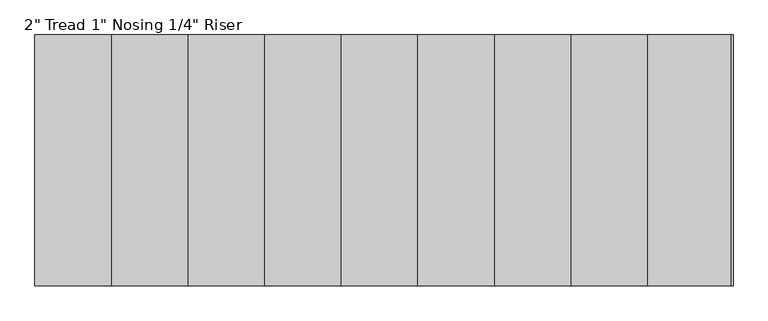
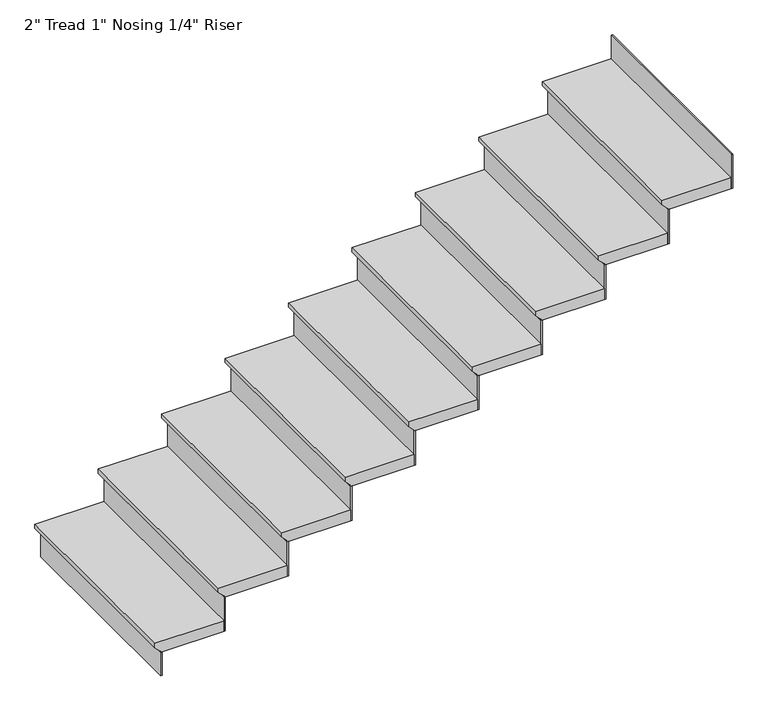
"""IFC4 building model written with IfcOpenShell, lengths in millimetres: stair flight geometry."""

from ifc_helpers import new_model, si_unit, origin, place, context, project, spatial, faceted_brep, source, transform, mapped, element, save


def stair_flight_ff2ce9cd(model_context):
    return source(origin(), model_context, "Body", "Brep", [
        faceted_brep([(-1591.1154463, -4737.3544725, 25744.17), (-1591.1154463, -4737.3544725, 25763.22), (-1591.1154463, -3822.9544725, 25763.22), (-1591.1154463, -3822.9544725, 25744.17), (-1565.7154463, -4737.3544725, 25718.77), (-1565.7154463, -3822.9544725, 25718.77), (-1286.3154463, -4737.3544725, 25763.22), (-1286.3154463, -3822.9544725, 25763.22), (-1565.7154463, -3822.9544725, 25712.42), (-1286.3154463, -3822.9544725, 25712.42), (-1286.3154463, -4737.3544725, 25712.42), (-1565.7154463, -4737.3544725, 25712.42)], [[[0, 1, 2, 3]], [[4, 0, 3, 5]], [[2, 1, 6, 7]], [[8, 9, 10, 11]], [[2, 7, 9, 8, 5, 3]], [[8, 11, 4, 5]], [[6, 1, 0, 4, 11, 10]], [[7, 6, 10, 9]]]),
        faceted_brep([(-1565.7154463, -4737.3544725, 25712.42), (-1565.7154463, -4737.3544725, 25603.2), (-1559.3654463, -4737.3544725, 25603.2), (-1559.3654463, -4737.3544725, 25712.42), (-1565.7154463, -3822.9544725, 25712.42), (-1559.3654463, -3822.9544725, 25712.42), (-1559.3654463, -3822.9544725, 25603.2), (-1565.7154463, -3822.9544725, 25603.2)], [[[0, 1, 2, 3]], [[4, 5, 6, 7]], [[1, 0, 4, 7]], [[2, 1, 7, 6]], [[3, 2, 6, 5]], [[0, 3, 5, 4]]]),
        faceted_brep([(-1286.3154463, -4737.3544725, 25872.44), (-1286.3154463, -4737.3544725, 25712.42), (-1279.9654463, -4737.3544725, 25712.42), (-1279.9654463, -4737.3544725, 25872.44), (-1286.3154463, -3822.9544725, 25872.44), (-1279.9654463, -3822.9544725, 25872.44), (-1279.9654463, -3822.9544725, 25712.42), (-1286.3154463, -3822.9544725, 25712.42)], [[[0, 1, 2, 3]], [[4, 5, 6, 7]], [[1, 0, 4, 7]], [[2, 1, 7, 6]], [[3, 2, 6, 5]], [[0, 3, 5, 4]]]),
        faceted_brep([(-1311.7154463, -3822.9544725, 25923.24), (-1311.7154463, -4737.3544725, 25923.24), (-1006.9154463, -4737.3544725, 25923.24), (-1006.9154463, -3822.9544725, 25923.24), (-1286.3154463, -3822.9544725, 25872.44), (-1006.9154463, -3822.9544725, 25872.44), (-1006.9154463, -4737.3544725, 25872.44), (-1286.3154463, -4737.3544725, 25872.44), (-1286.3154463, -3822.9544725, 25878.79), (-1311.7154463, -3822.9544725, 25904.19), (-1286.3154463, -4737.3544725, 25878.79), (-1311.7154463, -4737.3544725, 25904.19)], [[[0, 1, 2, 3]], [[4, 5, 6, 7]], [[0, 3, 5, 4, 8, 9]], [[4, 7, 10, 8]], [[2, 1, 11, 10, 7, 6]], [[3, 2, 6, 5]], [[11, 1, 0, 9]], [[10, 11, 9, 8]]]),
        faceted_brep([(-1006.9154463, -4737.3544725, 26032.46), (-1006.9154463, -4737.3544725, 25872.44), (-1000.5654463, -4737.3544725, 25872.44), (-1000.5654463, -4737.3544725, 26032.46), (-1006.9154463, -3822.9544725, 26032.46), (-1000.5654463, -3822.9544725, 26032.46), (-1000.5654463, -3822.9544725, 25872.44), (-1006.9154463, -3822.9544725, 25872.44)], [[[0, 1, 2, 3]], [[4, 5, 6, 7]], [[1, 0, 4, 7]], [[2, 1, 7, 6]], [[3, 2, 6, 5]], [[0, 3, 5, 4]]]),
        faceted_brep([(-1032.3154463, -3822.9544725, 26083.26), (-1032.3154463, -4737.3544725, 26083.26), (-727.5154463, -4737.3544725, 26083.26), (-727.5154463, -3822.9544725, 26083.26), (-1006.9154463, -3822.9544725, 26032.46), (-727.5154463, -3822.9544725, 26032.46), (-727.5154463, -4737.3544725, 26032.46), (-1006.9154463, -4737.3544725, 26032.46), (-1006.9154463, -3822.9544725, 26038.81), (-1032.3154463, -3822.9544725, 26064.21), (-1006.9154463, -4737.3544725, 26038.81), (-1032.3154463, -4737.3544725, 26064.21)], [[[0, 1, 2, 3]], [[4, 5, 6, 7]], [[0, 3, 5, 4, 8, 9]], [[4, 7, 10, 8]], [[2, 1, 11, 10, 7, 6]], [[3, 2, 6, 5]], [[11, 1, 0, 9]], [[10, 11, 9, 8]]]),
        faceted_brep([(-727.5154463, -4737.3544725, 26192.48), (-727.5154463, -4737.3544725, 26032.46), (-721.1654463, -4737.3544725, 26032.46), (-721.1654463, -4737.3544725, 26192.48), (-727.5154463, -3822.9544725, 26192.48), (-721.1654463, -3822.9544725, 26192.48), (-721.1654463, -3822.9544725, 26032.46), (-727.5154463, -3822.9544725, 26032.46)], [[[0, 1, 2, 3]], [[4, 5, 6, 7]], [[1, 0, 4, 7]], [[2, 1, 7, 6]], [[3, 2, 6, 5]], [[0, 3, 5, 4]]]),
        faceted_brep([(-752.9154463, -3822.9544725, 26243.28), (-752.9154463, -4737.3544725, 26243.28), (-448.1154463, -4737.3544725, 26243.28), (-448.1154463, -3822.9544725, 26243.28), (-727.5154463, -3822.9544725, 26192.48), (-448.1154463, -3822.9544725, 26192.48), (-448.1154463, -4737.3544725, 26192.48), (-727.5154463, -4737.3544725, 26192.48), (-727.5154463, -3822.9544725, 26198.83), (-752.9154463, -3822.9544725, 26224.23), (-727.5154463, -4737.3544725, 26198.83), (-752.9154463, -4737.3544725, 26224.23)], [[[0, 1, 2, 3]], [[4, 5, 6, 7]], [[0, 3, 5, 4, 8, 9]], [[4, 7, 10, 8]], [[2, 1, 11, 10, 7, 6]], [[3, 2, 6, 5]], [[11, 1, 0, 9]], [[10, 11, 9, 8]]]),
        faceted_brep([(-448.1154463, -4737.3544725, 26352.5), (-448.1154463, -4737.3544725, 26192.48), (-441.7654463, -4737.3544725, 26192.48), (-441.7654463, -4737.3544725, 26352.5), (-448.1154463, -3822.9544725, 26352.5), (-441.7654463, -3822.9544725, 26352.5), (-441.7654463, -3822.9544725, 26192.48), (-448.1154463, -3822.9544725, 26192.48)], [[[0, 1, 2, 3]], [[4, 5, 6, 7]], [[1, 0, 4, 7]], [[2, 1, 7, 6]], [[3, 2, 6, 5]], [[0, 3, 5, 4]]]),
        faceted_brep([(-473.5154463, -3822.9544725, 26403.3), (-473.5154463, -4737.3544725, 26403.3), (-168.7154463, -4737.3544725, 26403.3), (-168.7154463, -3822.9544725, 26403.3), (-448.1154463, -3822.9544725, 26352.5), (-168.7154463, -3822.9544725, 26352.5), (-168.7154463, -4737.3544725, 26352.5), (-448.1154463, -4737.3544725, 26352.5), (-448.1154463, -3822.9544725, 26358.85), (-473.5154463, -3822.9544725, 26384.25), (-448.1154463, -4737.3544725, 26358.85), (-473.5154463, -4737.3544725, 26384.25)], [[[0, 1, 2, 3]], [[4, 5, 6, 7]], [[0, 3, 5, 4, 8, 9]], [[4, 7, 10, 8]], [[2, 1, 11, 10, 7, 6]], [[3, 2, 6, 5]], [[11, 1, 0, 9]], [[10, 11, 9, 8]]]),
        faceted_brep([(-168.7154463, -4737.3544725, 26512.52), (-168.7154463, -4737.3544725, 26352.5), (-162.3654463, -4737.3544725, 26352.5), (-162.3654463, -4737.3544725, 26512.52), (-168.7154463, -3822.9544725, 26512.52), (-162.3654463, -3822.9544725, 26512.52), (-162.3654463, -3822.9544725, 26352.5), (-168.7154463, -3822.9544725, 26352.5)], [[[0, 1, 2, 3]], [[4, 5, 6, 7]], [[1, 0, 4, 7]], [[2, 1, 7, 6]], [[3, 2, 6, 5]], [[0, 3, 5, 4]]]),
        faceted_brep([(-194.1154463, -3822.9544725, 26563.32), (-194.1154463, -4737.3544725, 26563.32), (110.6845537, -4737.3544725, 26563.32), (110.6845537, -3822.9544725, 26563.32), (-168.7154463, -3822.9544725, 26512.52), (110.6845537, -3822.9544725, 26512.52), (110.6845537, -4737.3544725, 26512.52), (-168.7154463, -4737.3544725, 26512.52), (-168.7154463, -3822.9544725, 26518.87), (-194.1154463, -3822.9544725, 26544.27), (-168.7154463, -4737.3544725, 26518.87), (-194.1154463, -4737.3544725, 26544.27)], [[[0, 1, 2, 3]], [[4, 5, 6, 7]], [[0, 3, 5, 4, 8, 9]], [[4, 7, 10, 8]], [[2, 1, 11, 10, 7, 6]], [[3, 2, 6, 5]], [[11, 1, 0, 9]], [[10, 11, 9, 8]]]),
        faceted_brep([(110.6845537, -4737.3544725, 26672.54), (110.6845537, -4737.3544725, 26512.52), (117.0345537, -4737.3544725, 26512.52), (117.0345537, -4737.3544725, 26672.54), (110.6845537, -3822.9544725, 26672.54), (117.0345537, -3822.9544725, 26672.54), (117.0345537, -3822.9544725, 26512.52), (110.6845537, -3822.9544725, 26512.52)], [[[0, 1, 2, 3]], [[4, 5, 6, 7]], [[1, 0, 4, 7]], [[2, 1, 7, 6]], [[3, 2, 6, 5]], [[0, 3, 5, 4]]]),
        faceted_brep([(85.2845537, -3822.9544725, 26723.34), (85.2845537, -4737.3544725, 26723.34), (390.0845537, -4737.3544725, 26723.34), (390.0845537, -3822.9544725, 26723.34), (110.6845537, -3822.9544725, 26672.54), (390.0845537, -3822.9544725, 26672.54), (390.0845537, -4737.3544725, 26672.54), (110.6845537, -4737.3544725, 26672.54), (110.6845537, -3822.9544725, 26678.89), (85.2845537, -3822.9544725, 26704.29), (110.6845537, -4737.3544725, 26678.89), (85.2845537, -4737.3544725, 26704.29)], [[[0, 1, 2, 3]], [[4, 5, 6, 7]], [[0, 3, 5, 4, 8, 9]], [[4, 7, 10, 8]], [[2, 1, 11, 10, 7, 6]], [[3, 2, 6, 5]], [[11, 1, 0, 9]], [[10, 11, 9, 8]]]),
        faceted_brep([(390.0845537, -4737.3544725, 26832.56), (390.0845537, -4737.3544725, 26672.54), (396.4345537, -4737.3544725, 26672.54), (396.4345537, -4737.3544725, 26832.56), (390.0845537, -3822.9544725, 26832.56), (396.4345537, -3822.9544725, 26832.56), (396.4345537, -3822.9544725, 26672.54), (390.0845537, -3822.9544725, 26672.54)], [[[0, 1, 2, 3]], [[4, 5, 6, 7]], [[1, 0, 4, 7]], [[2, 1, 7, 6]], [[3, 2, 6, 5]], [[0, 3, 5, 4]]]),
        faceted_brep([(364.6845537, -3822.9544725, 26883.36), (364.6845537, -4737.3544725, 26883.36), (669.4845537, -4737.3544725, 26883.36), (669.4845537, -3822.9544725, 26883.36), (390.0845537, -3822.9544725, 26832.56), (669.4845537, -3822.9544725, 26832.56), (669.4845537, -4737.3544725, 26832.56), (390.0845537, -4737.3544725, 26832.56), (390.0845537, -3822.9544725, 26838.91), (364.6845537, -3822.9544725, 26864.31), (390.0845537, -4737.3544725, 26838.91), (364.6845537, -4737.3544725, 26864.31)], [[[0, 1, 2, 3]], [[4, 5, 6, 7]], [[0, 3, 5, 4, 8, 9]], [[4, 7, 10, 8]], [[2, 1, 11, 10, 7, 6]], [[3, 2, 6, 5]], [[11, 1, 0, 9]], [[10, 11, 9, 8]]]),
        faceted_brep([(948.8845537, -4737.3544725, 27152.6), (948.8845537, -4737.3544725, 26992.58), (955.2345537, -4737.3544725, 26992.58), (955.2345537, -4737.3544725, 27152.6), (948.8845537, -3822.9544725, 27152.6), (955.2345537, -3822.9544725, 27152.6), (955.2345537, -3822.9544725, 26992.58), (948.8845537, -3822.9544725, 26992.58)], [[[0, 1, 2, 3]], [[4, 5, 6, 7]], [[1, 0, 4, 7]], [[2, 1, 7, 6]], [[3, 2, 6, 5]], [[0, 3, 5, 4]]]),
        faceted_brep([(669.4845537, -4737.3544725, 26992.58), (669.4845537, -4737.3544725, 26832.56), (675.8345537, -4737.3544725, 26832.56), (675.8345537, -4737.3544725, 26992.58), (669.4845537, -3822.9544725, 26992.58), (675.8345537, -3822.9544725, 26992.58), (675.8345537, -3822.9544725, 26832.56), (669.4845537, -3822.9544725, 26832.56)], [[[0, 1, 2, 3]], [[4, 5, 6, 7]], [[1, 0, 4, 7]], [[2, 1, 7, 6]], [[3, 2, 6, 5]], [[0, 3, 5, 4]]]),
        faceted_brep([(948.8845537, -3822.9544725, 27043.38), (923.4845537, -3822.9544725, 27043.38), (644.0845537, -3822.9544725, 27043.38), (644.0845537, -4737.3544725, 27043.38), (948.8845537, -4737.3544725, 27043.38), (923.4845537, -3822.9544725, 26992.58), (948.8845537, -3822.9544725, 26992.58), (948.8845537, -4737.3544725, 26992.58), (669.4845537, -4737.3544725, 26992.58), (669.4845537, -3822.9544725, 26992.58), (669.4845537, -3822.9544725, 26998.93), (644.0845537, -3822.9544725, 27024.33), (669.4845537, -4737.3544725, 26998.93), (644.0845537, -4737.3544725, 27024.33)], [[[0, 1, 2, 3, 4]], [[5, 6, 7, 8, 9]], [[1, 0, 6, 5]], [[2, 1, 5, 9, 10, 11]], [[9, 8, 12, 10]], [[4, 3, 13, 12, 8, 7]], [[0, 4, 7, 6]], [[13, 3, 2, 11]], [[12, 13, 11, 10]]]),
    ])


if __name__ == "__main__":
    model = new_model("IFC4")
    model_context = context("Model", 3, world=origin())
    ifc_project = project(units=[si_unit("LENGTHUNIT", "METRE", prefix="MILLI")], contexts=[model_context])
    site = spatial("IfcSite", under=ifc_project)
    building = spatial("IfcBuilding", under=site)
    placement = place(None, origin())
    stair_flight_shape = stair_flight_ff2ce9cd(model_context)
    element("IfcStairFlight", 1, ObjectType="2\" Tread 1\" Nosing 1/4\" Riser", at=placement, inside=building, context=model_context, shape_type="MappedRepresentation", body=[
        mapped(stair_flight_shape, transform((0.0, 0.0, 0.0), x_axis=(1.0, 0.0, 0.0), y_axis=(0.0, 1.0, 0.0), z_axis=(0.0, 0.0, 1.0))),
    ])
    save(model, "model.ifc")
